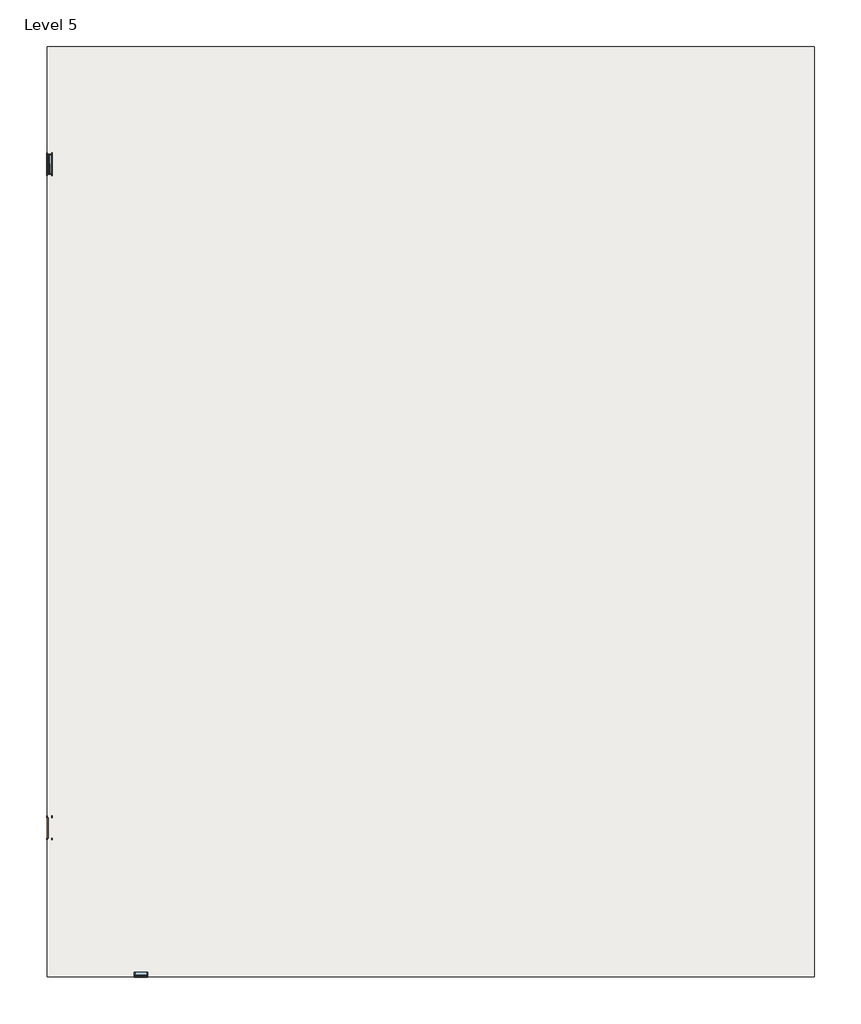
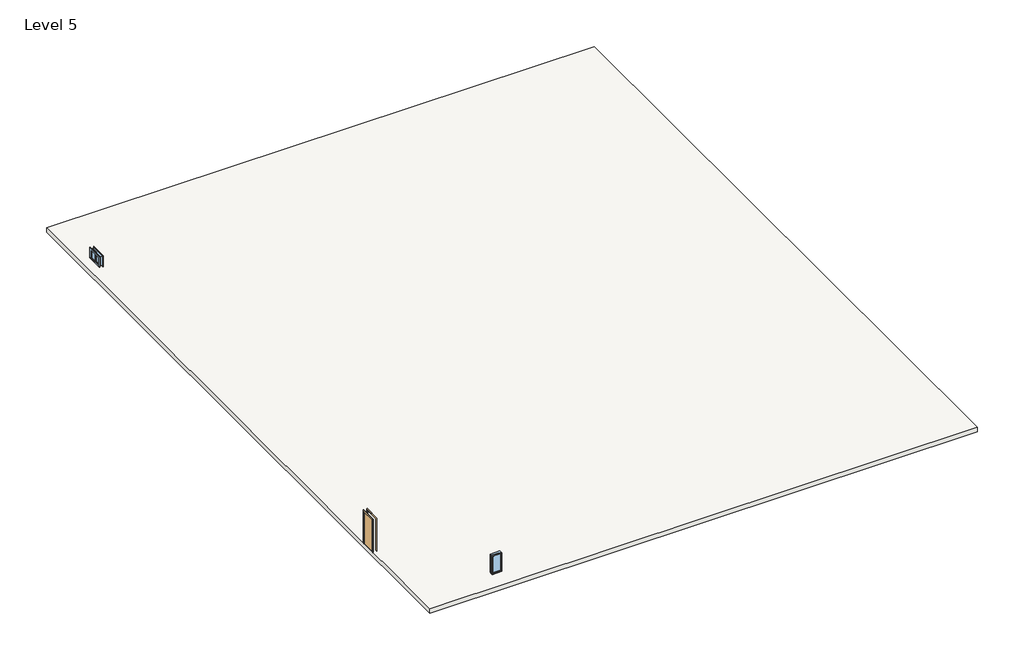
# One storey: 2 windows, 1 door, 1 slab.
"""IFC4 building model written with IfcOpenShell, lengths in millimetres."""

from ifc_helpers import new_model, si_unit, frame, origin, place, context, project, spatial, polyline, outline, extrude, transform, mapped, element, save
from components import door_54dd4da4, window_78885257, window_a4355bb3

model = new_model("IFC4")

# Units and contexts
model_context = context("Model", 3, world=origin())
ifc_project = project(units=[si_unit("LENGTHUNIT", "METRE", prefix="MILLI")], contexts=[model_context])

# Site, building, storey
site = spatial("IfcSite", under=ifc_project)
building = spatial("IfcBuilding", under=site)
storey = spatial("IfcBuildingStorey", under=building, Name="Level 5", Elevation=9448.8)

# Door
placement = place(None, origin())
door_shape = door_54dd4da4(model_context)
element("IfcDoor", 1, ObjectType="Single-Flush : 36\" x 84\"", at=placement, inside=storey, context=model_context, shape_type="MappedRepresentation", body=[
    mapped(door_shape, transform((-15175.038074, -14157.3915889, 9448.8), x_axis=(0.0, 1.0, 0.0), y_axis=(-1.0, 0.0, 0.0), z_axis=(0.0, 0.0, 1.0))),
])

# Slab
element("IfcSlab", 2, ObjectType="Generic - 12\"", at=placement, inside=storey, context=model_context, shape_type="SweptSolid", body=[
    extrude(outline(polyline([(19165.761926, 20911.8014639), (19165.761926, -20845.7985361), (-15276.638074, -20845.7985361), (-15276.638074, 20911.8014639), (19165.761926, 20911.8014639)])), frame((0.0, 0.0, 9144.0), z_axis=(0.0, 0.0, 1.0), x_axis=(1.0, 0.0, 0.0)), (0.0, 0.0, 1.0), 304.8),
])

# Windows
window_shape = window_78885257(model_context)
element("IfcWindow", 3, ObjectType="Instance - Fixed : 24\" x 48\"", at=placement, inside=storey, context=model_context, shape_type="MappedRepresentation", body=[
    mapped(window_shape, transform((-11098.338074, -20744.1985361, 9448.8), x_axis=(-1.0, 0.0, 0.0), y_axis=(0.0, -1.0, 0.0), z_axis=(0.0, 0.0, 1.0))),
])
window_2_shape = window_a4355bb3(model_context)
element("IfcWindow", 4, ObjectType="Slider with Trim : 36\" x 24\"", at=placement, inside=storey, context=model_context, shape_type="MappedRepresentation", body=[
    mapped(window_2_shape, transform((-15175.038074, 15628.6014639, 9448.8), x_axis=(0.0, 1.0, 0.0), y_axis=(-1.0, 0.0, 0.0), z_axis=(0.0, 0.0, 1.0))),
])

save(model, "model.ifc")

# Revit data of these elements
# Type "Single-Flush : 36\" x 84\""
#   Type Mark = "1"
#   Construction Type Id = "MDOOR"
#   Assembly Code = "C1020"
#   Analytic Construction = "Metal"
#   Thickness = 0' - 2"
#   Heat Transfer Coefficient (U) = 0.651978 BTU/(h·ft²·°F)
#   Height = 7' - 0"
#   Trim Projection Ext = 0' - 1"
#   Trim Projection Int = 0' - 1"
#   Trim Width = 0' - 3"
#   Width = 3' - 0"
#   Define Thermal Properties by = 1
#   Door Material = Door - Panel
#   Frame Material = Door - Frame
#   Visual Light Transmittance = 0
#   Solar Heat Gain Coefficient = 0
#   Function = (empty or 0)
#   Wall Closure = (empty or 0)
# Type "Generic - 12\""
#   Assembly Code = "B1010"
#   Function = 0
#   Layers, outside or top first: 1' - 0" no material (function 1)
# Type "Instance - Fixed : 24\" x 48\""
#   Type Mark = "19"
#   Construction Type Id = "GSP4R"
#   Assembly Code = "B2020100"
#   Analytic Construction = "1/8 in Pilkington single glazing"
#   Visual Light Transmittance = 0.9
#   Thermal Resistance (R) = 0.8466 (h·ft²·°F)/BTU
#   Solar Heat Gain Coefficient = 0.86
#   Heat Transfer Coefficient (U) = 1.1812 BTU/(h·ft²·°F)
#   Height [instance default] = 4' - 0"
#   Default Sill Height = 3' - 0"
#   Width [instance default] = 2' - 0"
#   Window Inset = 0' - 0 3/4"
#   Define Thermal Properties by = 1
#   Glass Pane Material = Glass
#   Sash Material = Sash
#   Wall Closure = (empty or 0)
# Type "Slider with Trim : 36\" x 24\""
#   Type Mark = "23"
#   Construction Type Id = "GSP4R"
#   Assembly Code = "B2020100"
#   Analytic Construction = "1/8 in Pilkington single glazing"
#   Visual Light Transmittance = 0.9
#   Solar Heat Gain Coefficient = 0.78
#   Heat Transfer Coefficient (U) = 0.6496 BTU/(h·ft²·°F)
#   Height = 2' - 0"
#   Default Sill Height = 3' - 0"
#   Trim Projection - Ext. = 0' - 0 3/4"
#   Trim Projection - Int. = 0' - 0 3/4"
#   Trim Width - Exterior = 0' - 3 1/2"
#   Trim Width - Interior = 0' - 3 1/2"
#   Width = 3' - 0"
#   Window Inset = 0' - 0 3/4"
#   Define Thermal Properties by = 1
#   Glass Pane Material = Glass
#   Sash Material = Sash
#   Trim Exterior Material = Trim
#   Trim Interior Material = Trim
#   Wall Closure = (empty or 0)
# Element 1 (IfcDoor, "Single-Flush : 36\" x 84\"")
#   Phase Created = New Construction
#   Materials on its faces: "Door - Frame", "Door - Panel"
# Element 2 (IfcSlab, "Generic - 12\"")
#   Height Offset From Level = 0' - 0"
#   Phase Created = New Construction
#   Materials on its faces: "Default Floor"
# Element 3 (IfcWindow, "Instance - Fixed : 24\" x 48\"")
#   Mark = "20"
#   Width = 2' - 0"
#   Height = 4' - 0"
#   Phase Created = New Construction
#   Materials on its faces: "Sash", "Glass"
# Element 4 (IfcWindow, "Slider with Trim : 36\" x 24\"")
#   Mark = "64"
#   Phase Created = New Construction
#   Materials on its faces: "Sash", "Trim", "Glass"
# Materials
#   "Door - Panel": class "Wood", colour RGB 210 159 95, transparency 0
#   "Door - Frame": colour RGB 118 70 51, transparency 0
#   "Glass": class "Glass", colour RGB 0 128 192, transparency 0.75, Description = "Soda Lime Glass", Cost = 0
#   "Sash": class "Wood", colour RGB 224 178 126, transparency 0
#   "Trim": class "Wood", colour RGB 224 178 126, transparency 0
#   "Default Floor": colour RGB 128 128 128, transparency 0
